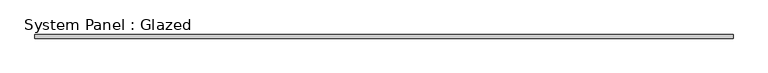
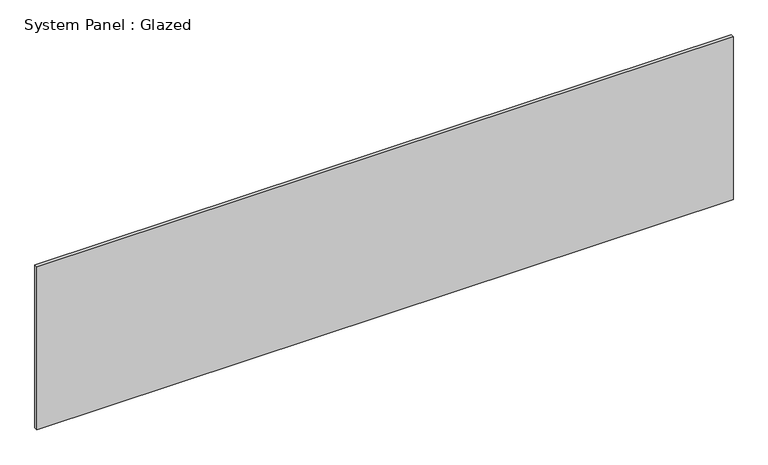
"""IFC4 building model written with IfcOpenShell, lengths in millimetres: plate geometry, System Panel : Glazed."""

from ifc_helpers import new_model, si_unit, origin, origin_with_axes, place, context, project, spatial, polyline, outline, extrude, source, transform, mapped, element, save


def system_panel_glazed_4d78ce51(model_context):
    return source(origin(), model_context, "Body", "SweptSolid", [
        extrude(outline(polyline([(2462.6390576, 19.05), (-2462.6390576, 19.05), (-2462.6390576, 44.45), (2462.6390576, 44.45), (2462.6390576, 19.05)])), origin_with_axes(), (0.0, 0.0, 1.0), 1219.2),
    ])


if __name__ == "__main__":
    model = new_model("IFC4")
    model_context = context("Model", 3, world=origin())
    ifc_project = project(units=[si_unit("LENGTHUNIT", "METRE", prefix="MILLI")], contexts=[model_context])
    site = spatial("IfcSite", under=ifc_project)
    building = spatial("IfcBuilding", under=site)
    placement = place(None, origin())
    system_panel_glazed_shape = system_panel_glazed_4d78ce51(model_context)
    element("IfcPlate", 1, ObjectType="System Panel : Glazed", at=placement, inside=building, context=model_context, shape_type="MappedRepresentation", body=[
        mapped(system_panel_glazed_shape, transform((0.0, 0.0, 0.0), x_axis=(1.0, 0.0, 0.0), y_axis=(0.0, 1.0, 0.0), z_axis=(0.0, 0.0, 1.0))),
    ])
    save(model, "model.ifc")

# Revit data of these elements
# Type "System Panel : Glazed"
#   Construction Type Id = "GSP4R"
#   Analytic Construction = "1/8 in Pilkington single glazing"
#   Visual Light Transmittance = 0.9
#   Solar Heat Gain Coefficient = 0.86
#   Heat Transfer Coefficient (U) = 1.18115 BTU/(h·ft²·°F)
# Element 1 (IfcPlate, "System Panel : Glazed")
#   Materials on its faces: "Glass"
# Materials
#   "Glass": class "Glass", colour RGB 0 128 192, transparency 0.75, Description = "Soda Lime Glass", Cost = 0
